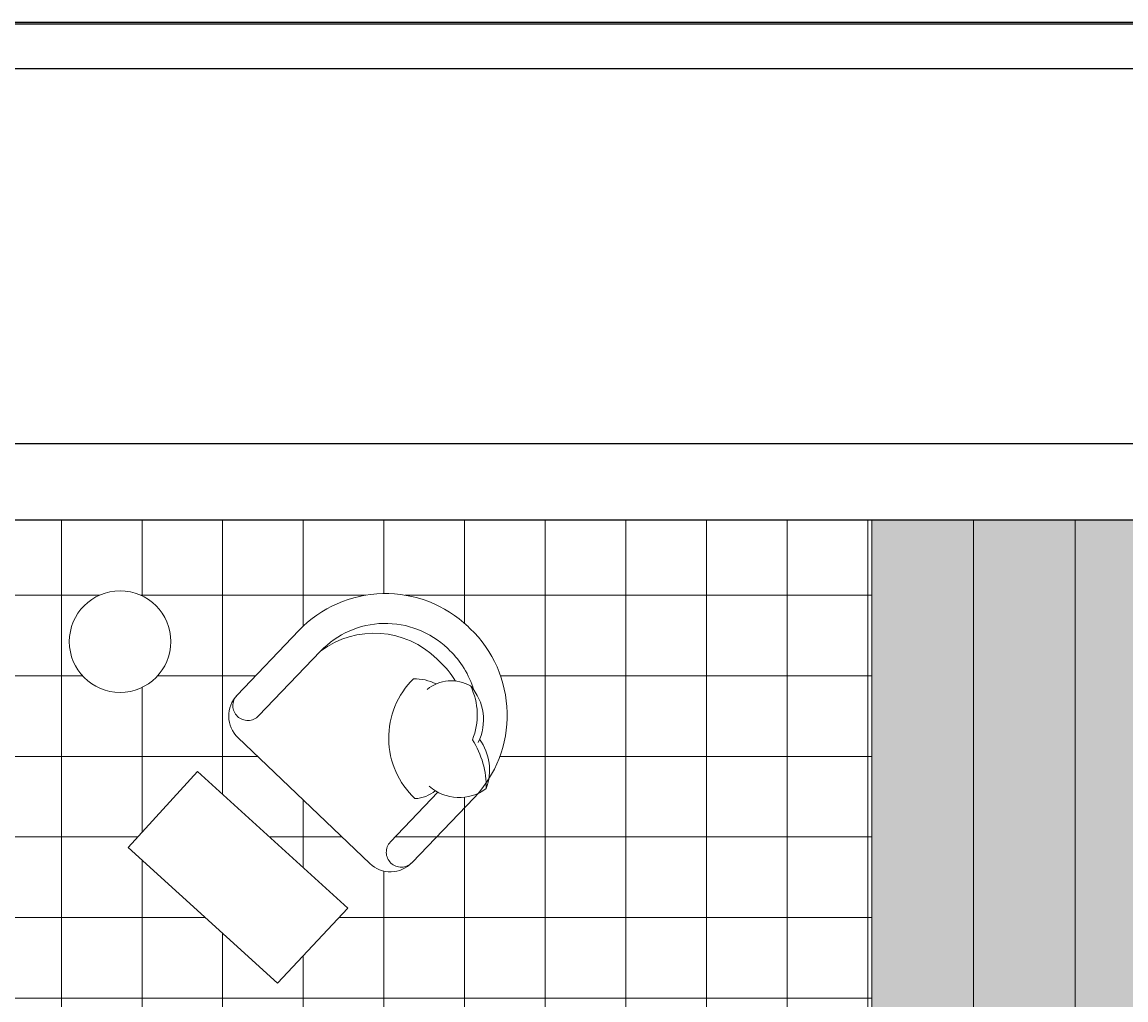
# Model space of a CAD drawing. Units: inches. Extents: x 84 to 1044, y -280 to 906.
# Tile 64 of 105: x 310 to 440, y 790 to 906. Entities that reach past the tile are written whole.
import ezdxf

# ---------------------------------------------------------------- set-up
doc = ezdxf.new("R2010")
doc.units = ezdxf.units.IN
for name, color, linetype, lineweight in [('A-ANNO-DIMS', 2, 'Continuous', 18), ('A-ANNO-TTLB', 7, 'Continuous', 25), ('A-FURN', 8, 'Continuous', 15), ('A-STAIRCASE', 144, 'Continuous', 18), ('C-PROP', 7, 'Continuous', 25)]:
    doc.layers.add(name, color=color, linetype=linetype, lineweight=lineweight)
for name, color, linetype, lineweight, true_color in [('A-FLOR-PATT', 251, 'Continuous', 9, 0x705861), ('A-FLOR-STRS-PATT', 35, 'Continuous', 9, 0x947764), ('L-PLNT-PATT', 9, 'Continuous', 9, 0xafd9aa)]:
    doc.layers.add(name, color=color, linetype=linetype, lineweight=lineweight, true_color=true_color)
doc.styles.get("Standard").update_dxf_attribs({"font": 'arial.ttf'})
doc.dimstyles.get("Standard").update_dxf_attribs({"dimtxt": 0.18, "dimasz": 0.18, "dimexe": 0.18, "dimexo": 0.0625, "dimgap": 0.09, "dimtad": 0, "dimtih": 1, "dimtoh": 1, "dimdec": 4, "dimzin": 0, "dimdsep": 46, "dimtxsty": 'Standard', "dimcen": 0.09, "dimadec": 0, "dimazin": 0, "dimtfac": 1, "dimtdec": 4, "dimtofl": 0, "dimtmove": 0, "dimatfit": 3, "dimfxl": 1, "dimtolj": 1, "dimtzin": 0, "dimarcsym": 0})

# ---------------------------------------------------------------- blocks, each defined once
blk = doc.blocks.new('*D62')
at = {"layer": 'A-ANNO-DIMS', "color": 0, "lineweight": -2, "transparency": 16777216}
for p, q in [((203.18, 709.18), (203.18, 905.9)), ((203.36, 905.72), (549.23, 905.72)), ((895.89, 905.72), (550.02, 905.72)), ((896.07, 400.18), (896.07, 905.9))]:
    blk.add_line(p, q, dxfattribs=at)
at = {"layer": 'A-ANNO-DIMS', "color": 0, "transparency": 16777216}
for points in [[(203.36, 905.75), (203.36, 905.69), (203.18, 905.72)], [(895.89, 905.75), (895.89, 905.69), (896.07, 905.72)]]:
    blk.add_solid(points, dxfattribs=at)
at = {"layer": 'Defpoints', "color": 0, "transparency": 16777216}
for p in [(896.07, 905.72), (203.18, 709.12), (896.07, 400.12)]:
    blk.add_point(p, dxfattribs=at)
at = {"layer": 'A-ANNO-DIMS', "color": 0, "transparency": 16777216, "insert": (549.63, 905.72), "char_height": 0.18, "attachment_point": 5}
blk.add_mtext('\\A1;692.9', dxfattribs=at)

msp = doc.modelspace()

# ---------------------------------------------------------------- hatches: boundary and pattern name
at = {"layer": 'A-FLOR-PATT', "transparency": 33554597}
h = msp.add_hatch(dxfattribs=at)
h.set_pattern_fill('ANSI37', color=256, scale=3, angle=45)
h.paths.add_polyline_path([(410.074, 847.12), (143.179, 847.12), (143.179, 769.12), (203.179, 769.12), (410.074, 769.12)])
h.paths.add_polyline_path([(254.313, 826.374, -0.4142136), (254.257, 823.878, -0.4142136), (251.76, 823.934), (244.439, 831.592, 0.3775004), (230.555, 830.526, 0.0765992), (228.51, 828.052, -0.127919), (230.803, 827.709, -0.1215233), (233.469, 828.328, -0.4259892), (233.291, 814.163, -0.1655406), (230.889, 815.094, -0.0168883), (230.578, 814.914), (236.189, 809.046, -0.4142136), (236.133, 806.549, -0.4142136), (233.636, 806.605, 0.4142136), (238.63, 806.493), (246.415, 813.937), (254.201, 821.381, 0.4142136)], flags=16)
h.paths.add_polyline_path([(241.241, 801.211), (258.998, 817.357), (267.168, 808.372), (249.545, 792.347)], flags=16)
h.paths.add_polyline_path([(262.121, 832.717, -1), (274.121, 832.717, -1)], flags=16)
h.paths.add_polyline_path([(315.269, 832.717, -1), (327.269, 832.717, -1)], flags=16)
h.paths.add_polyline_path([(322.221, 808.372), (330.392, 817.357), (348.148, 801.211), (339.844, 792.347)], flags=16)
h.paths.add_polyline_path([(344.951, 831.592, -0.3727189), (358.711, 830.652), (358.966, 830.408, -0.0723842), (360.879, 828.052, -0.1030417), (362.667, 827.476, -0.0234196), (363.022, 827.039, 0.1348317), (360.058, 831.805, 0.4191038)], flags=0)
h.paths.add_polyline_path([(355.753, 806.605, -0.4142136), (353.257, 806.549, -0.4142136), (353.201, 809.046), (358.811, 814.914, 0.2341585), (363.536, 814.769, 0.4037218), (362.499, 834.358, 0.4178796), (342.398, 834.032), (335.076, 826.374, 0.4142136), (335.188, 821.381), (342.974, 813.937), (350.76, 806.493, 0.4142136)], flags=16)
at = {"layer": 'A-FLOR-STRS-PATT', "transparency": 33554567}
h = msp.add_hatch(color=256, dxfattribs=at)
h.dxf.hatch_style = 1
h.paths.add_polyline_path([(650.074, 91.12), (638.074, 91.12), (638.074, 67.12), (455.074, 67.12), (455.074, 55.12), (650.074, 55.12)], flags=17)
h.paths.add_polyline_path([(662.074, 91.12), (650.074, 91.12), (650.074, 55.12), (455.074, 55.12), (455.074, 43.12), (662.074, 43.12)])
h.paths.add_polyline_path([(674.074, 91.12), (671.074, 91.12), (662.074, 91.12), (662.074, 43.12), (455.074, 43.12), (455.074, 31.12), (674.074, 31.12)])
h.paths.add_polyline_path([(227.179, 151.12), (203.179, 151.12), (143.179, 151.12), (143.179, 139.12), (227.179, 139.12)])
h.paths.add_polyline_path([(227.179, 139.12), (143.179, 139.12), (143.179, 127.12), (227.179, 127.12)])
h.paths.add_polyline_path([(203.179, 271.12), (143.179, 271.12), (143.179, 259.12), (203.179, 259.12)])
h.paths.add_polyline_path([(203.179, 259.12), (143.179, 259.12), (143.179, 247.12), (203.179, 247.12)])
h.paths.add_polyline_path([(203.179, 769.12), (143.179, 769.12), (143.179, 757.12), (203.179, 757.12)])
h.paths.add_polyline_path([(203.179, 757.12), (143.179, 757.12), (143.179, 745.12), (203.179, 745.12)])
h.paths.add_polyline_path([(434.074, 847.12), (422.074, 847.12), (422.074, 769.12), (434.074, 769.12)])
h.paths.add_polyline_path([(422.074, 847.12), (410.074, 847.12), (410.074, 769.12), (422.074, 769.12)])
at = {"layer": 'L-PLNT-PATT', "transparency": 33554597}
h = msp.add_hatch(color=256, dxfattribs=at)
h.dxf.hatch_style = 1
h.paths.add_polyline_path([(434.074, 769.12), (386.074, 769.12), (386.074, 709.12), (434.074, 709.12)])
h.paths.add_polyline_path([(896.074, 847.12), (434.074, 847.12), (434.074, 769.12), (434.074, 709.12), (470.074, 709.12), (506.074, 709.12), (572.074, 709.12), (608.074, 709.12), (698.074, 709.12), (770.074, 709.12), (833.074, 709.12), (896.074, 709.12)])
h.paths.add_polyline_path([(983.074, 847.12), (896.074, 847.12), (896.074, 709.12), (896.074, 547.12), (932.074, 547.12), (983.074, 547.12)])
h.paths.add_polyline_path([(983.074, 547.12), (932.074, 547.12), (932.074, 265.12), (983.074, 265.12)])
h.paths.add_polyline_path([(203.179, 646.12), (203.179, 709.12), (203.179, 745.12), (143.179, 745.12), (143.179, 271.12), (203.179, 271.12), (203.179, 274.12), (203.179, 310.12), (203.179, 574.12)])

# ---------------------------------------------------------------- linework, layer by layer
at = {"layer": 'A-ANNO-TTLB'}
for points in [[(101.1, 905.916), (1027.308, 905.916), (1027.308, -279.764), (101.1, -279.764)], [(106.576, 900.439), (1021.832, 900.439), (1021.832, -274.288), (106.576, -274.288)]]:
    msp.add_lwpolyline(points, close=True, dxfattribs=at)
at = {"layer": 'A-FURN'}
for points in [[(342.974, 813.937), (335.188, 821.381, -0.4142136), (335.076, 826.374), (342.398, 834.032, -0.4142136), (362.372, 834.481), (362.499, 834.359), (362.627, 834.237, -0.4142136), (363.075, 814.263), (355.753, 806.605, -0.4142136), (350.76, 806.493), (342.974, 813.937)], [(344.951, 831.592, -0.4142136), (359.931, 831.928), (360.059, 831.806)], [(344.951, 831.592, -0.3727189), (358.711, 830.652), (358.838, 830.53)], [(344.951, 831.592), (337.629, 823.934, -0.4142136), (335.132, 823.878), (335.132, 823.878, -0.4142136), (335.076, 826.374)], [(363.022, 827.039, 0.1305915), (360.186, 831.684), (360.059, 831.806)], [(360.879, 828.052, 0.0723842), (358.966, 830.408), (358.838, 830.53)], [(358.5, 815.094, -0.1655406), (356.098, 814.163, -0.4259892), (355.921, 828.328, -0.1215233), (358.586, 827.709, 7.1154643)], [(363.565, 820.794, 0.3066635), (362.667, 827.476, 0.30633), (357.524, 827.076, -0.8728472)], [(364.516, 815.352, 0.1477299), (362.883, 821.112, 0.2133428), (362.667, 827.476, 0.1786618)], [(357.783, 815.632, 0.3567724), (364.516, 815.352, 0.2495421), (363.737, 821.172, -9.6168803)], [(358.811, 814.914), (353.201, 809.046, 0.4142136), (353.257, 806.549), (353.257, 806.549, 0.4142136), (355.753, 806.605)]]:
    msp.add_lwpolyline(points, format="xyb", dxfattribs=at)
msp.add_lwpolyline([(330.392, 817.357), (322.221, 808.372), (339.844, 792.347), (348.148, 801.211)], close=True, dxfattribs=at)
msp.add_circle((321.269, 832.717), 6, dxfattribs=at)
at = {"layer": 'A-STAIRCASE'}
for p, q in [((410.074, 769.12), (410.074, 847.12)), ((422.074, 769.12), (422.074, 847.12)), ((434.074, 769.12), (434.074, 847.12))]:
    msp.add_line(p, q, dxfattribs=at)
at = {"layer": 'C-PROP'}
for points in [[(143.179, -121.88), (134.179, -121.88), (134.179, 856.12), (992.074, 856.12), (992.074, -121.88), (624.574, -121.88)], [(143.179, -112.88), (143.179, 847.12), (983.074, 847.12), (983.074, -112.88), (624.574, -112.88)]]:
    msp.add_lwpolyline(points, dxfattribs=at)

# ---------------------------------------------------------------- dimensions: what is measured, and where the dimension line sits
at = {"layer": 'A-ANNO-DIMS'}
dim = msp.add_linear_dim(base=(896.074, 905.72), p1=(203.179, 709.12), p2=(896.074, 400.12), dimstyle='Standard', override={"dimdec": 1, "dimlfac": 1, "dimrnd": 0, "dimzin": 0, "dimdsep": 46, "dimlunit": 2}, dxfattribs=at)
dim.commit()
dim.dimension.update_dxf_attribs({"geometry": '*D62', "text_midpoint": (549.627, 905.72)})

doc.saveas('drawing.dxf')
